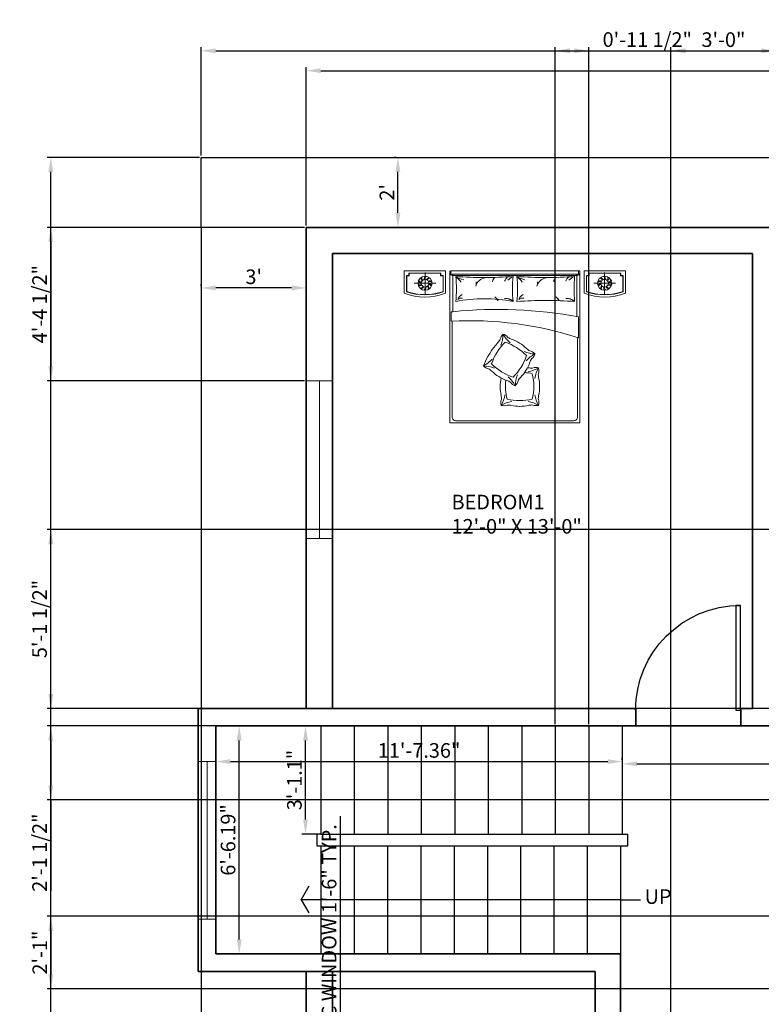
# Model space of a CAD drawing. Units: inches. Extents: x -938 to -211, y -366 to 366.
# Tile 2 of 4: x -938 to -684, y 4 to 341. Entities that reach past the tile are written whole.
import ezdxf

# ---------------------------------------------------------------- set-up
doc = ezdxf.new("R2010")
doc.units = ezdxf.units.IN
doc.header["$PDMODE"] = 35
doc.header["$PDSIZE"] = 5
for name, color, linetype, lineweight in [('A-ANNO-DIMS', 2, 'Continuous', 18), ('A-AREA-IDEN', 7, 'Continuous', 18), ('A-DOOR', 3, 'Continuous', 25), ('A-FLOR-STRS', 7, 'Continuous', 25), ('A-GLAZ', 4, 'Continuous', 18), ('A-WALL', 7, 'Continuous', 35), ('C-PROP', 8, 'Continuous', 25), ('furn', 28, 'Continuous', 13), ('txt', 7, 'Continuous', 18)]:
    doc.layers.add(name, color=color, linetype=linetype, lineweight=lineweight)
doc.styles.get("Standard").update_dxf_attribs({"font": 'arial.ttf'})
doc.dimstyles.new('ISO-25', dxfattribs={"dimtxt": 5, "dimasz": 5, "dimexe": 1.25, "dimexo": 0.625, "dimtad": 1, "dimlunit": 3, "dimtxsty": 'Standard', "dimcen": 2.5, "dimadec": 0, "dimazin": 0, "dimtfac": 1, "dimtmove": 0, "dimatfit": 3, "dimfxl": 1, "dimarcsym": 0})

# ---------------------------------------------------------------- blocks, each defined once
blk = doc.blocks.new('*U2')
for p, q in [((0, 0), (0, -6)), ((40, 0), (40, -6))]:
    blk.add_line(p, q)
blk.add_lwpolyline([(0, 0), (0, 40), (1.75, 40), (1.75, 0)], close=True)
blk.add_arc((0, 0), 40, 0, 90)
blk = doc.blocks.new('*D14')
at = {"layer": 'A-ANNO-DIMS', "color": 0, "lineweight": -2, "transparency": 16777216}
for p, q in [((-560.06, 104.36), (-560.06, 84.74)), ((-731.7, 98.36), (-731.7, 84.74)), ((-726.7, 85.99), (-565.06, 85.99))]:
    blk.add_line(p, q, dxfattribs=at)
at = {"layer": 'A-ANNO-DIMS', "color": 0, "transparency": 16777216}
for points in [[(-726.7, 86.82), (-726.7, 85.15), (-731.7, 85.99)], [(-565.06, 86.82), (-565.06, 85.15), (-560.06, 85.99)]]:
    blk.add_solid(points, dxfattribs=at)
at = {"layer": 'Defpoints', "color": 0, "transparency": 16777216}
for p in [(-560.06, 104.98), (-731.7, 98.98), (-560.06, 85.99)]:
    blk.add_point(p, dxfattribs=at)
at = {"layer": 'A-ANNO-DIMS', "color": 0, "transparency": 16777216, "insert": (-645.88, 89.17), "char_height": 5, "attachment_point": 5}
blk.add_mtext('14\'-3.64"', dxfattribs=at)
blk = doc.blocks.new('*D15')
at = {"layer": 'A-ANNO-DIMS', "color": 0, "lineweight": -2, "transparency": 16777216}
for p, q in [((-870.44, 98.98), (-861.78, 98.98)), ((-863.03, 25.79), (-863.03, 93.98)), ((-870.44, 20.79), (-861.78, 20.79))]:
    blk.add_line(p, q, dxfattribs=at)
at = {"layer": 'A-ANNO-DIMS', "color": 0, "transparency": 16777216}
for points in [[(-863.87, 93.98), (-862.2, 93.98), (-863.03, 98.98)], [(-863.87, 25.79), (-862.2, 25.79), (-863.03, 20.79)]]:
    blk.add_solid(points, dxfattribs=at)
at = {"layer": 'Defpoints', "color": 0, "transparency": 16777216}
for p in [(-871.06, 98.98), (-863.03, 98.98), (-871.06, 20.79)]:
    blk.add_point(p, dxfattribs=at)
at = {"layer": 'A-ANNO-DIMS', "color": 0, "transparency": 16777216, "insert": (-866.21, 59.89), "char_height": 5, "attachment_point": 5, "rotation": 90}
blk.add_mtext('6\'-6.19"', dxfattribs=at)
blk = doc.blocks.new('*D16')
at = {"layer": 'A-ANNO-DIMS', "color": 0, "lineweight": -2, "transparency": 16777216}
for p, q in [((-835.69, 98.98), (-841.54, 98.98)), ((-840.29, 66.89), (-840.29, 93.98)), ((-836.19, 61.89), (-841.54, 61.89))]:
    blk.add_line(p, q, dxfattribs=at)
at = {"layer": 'A-ANNO-DIMS', "color": 0, "transparency": 16777216}
for points in [[(-841.12, 93.98), (-839.46, 93.98), (-840.29, 98.98)], [(-841.12, 66.89), (-839.46, 66.89), (-840.29, 61.89)]]:
    blk.add_solid(points, dxfattribs=at)
at = {"layer": 'Defpoints', "color": 0, "transparency": 16777216}
for p in [(-840.29, 98.98), (-835.06, 98.98), (-835.56, 61.89)]:
    blk.add_point(p, dxfattribs=at)
at = {"layer": 'A-ANNO-DIMS', "color": 0, "transparency": 16777216, "insert": (-843.47, 80.43), "char_height": 5, "attachment_point": 5, "rotation": 90}
blk.add_mtext('3\'-1.1"', dxfattribs=at)
blk = doc.blocks.new('*D17')
at = {"layer": 'A-ANNO-DIMS', "color": 0, "lineweight": -2, "transparency": 16777216}
for p, q in [((-871.06, 87.39), (-871.06, 88.01)), ((-731.7, 87.39), (-731.7, 88.01)), ((-866.06, 86.76), (-736.7, 86.76))]:
    blk.add_line(p, q, dxfattribs=at)
at = {"layer": 'A-ANNO-DIMS', "color": 0, "transparency": 16777216}
for points in [[(-866.06, 87.59), (-866.06, 85.93), (-871.06, 86.76)], [(-736.7, 87.59), (-736.7, 85.93), (-731.7, 86.76)]]:
    blk.add_solid(points, dxfattribs=at)
at = {"layer": 'Defpoints', "color": 0, "transparency": 16777216}
for p in [(-871.06, 86.76), (-731.7, 86.76), (-731.7, 86.76)]:
    blk.add_point(p, dxfattribs=at)
at = {"layer": 'A-ANNO-DIMS', "color": 0, "transparency": 16777216, "insert": (-801.38, 89.94), "char_height": 5, "attachment_point": 5}
blk.add_mtext('11\'-7.36"', dxfattribs=at)
blk = doc.blocks.new('*D20')
at = {"layer": 'A-ANNO-DIMS', "color": 0, "lineweight": -2, "transparency": 16777216}
for p, q in [((-809.24, 293.98), (-809.87, 293.98)), ((-808.62, 274.98), (-808.62, 288.98)), ((-809.24, 269.98), (-809.87, 269.98))]:
    blk.add_line(p, q, dxfattribs=at)
at = {"layer": 'A-ANNO-DIMS', "color": 0, "transparency": 16777216}
for points in [[(-809.45, 288.98), (-807.78, 288.98), (-808.62, 293.98)], [(-809.45, 274.98), (-807.78, 274.98), (-808.62, 269.98)]]:
    blk.add_solid(points, dxfattribs=at)
at = {"layer": 'Defpoints', "color": 0, "transparency": 16777216}
for p in [(-808.62, 293.98), (-808.62, 293.98), (-808.62, 269.98)]:
    blk.add_point(p, dxfattribs=at)
at = {"layer": 'A-ANNO-DIMS', "color": 0, "transparency": 16777216, "insert": (-811.75, 281.98), "char_height": 5, "attachment_point": 5, "rotation": 90}
blk.add_mtext("2'", dxfattribs=at)
blk = doc.blocks.new('*D21')
at = {"layer": 'A-ANNO-DIMS', "color": 0, "lineweight": -2, "transparency": 16777216}
for p, q in [((-876.06, 249.82), (-876.06, 250.45)), ((-840.06, 249.82), (-840.06, 250.45)), ((-845.06, 249.2), (-871.06, 249.2))]:
    blk.add_line(p, q, dxfattribs=at)
at = {"layer": 'A-ANNO-DIMS', "color": 0, "transparency": 16777216}
for points in [[(-871.06, 250.03), (-871.06, 248.37), (-876.06, 249.2)], [(-845.06, 250.03), (-845.06, 248.37), (-840.06, 249.2)]]:
    blk.add_solid(points, dxfattribs=at)
at = {"layer": 'Defpoints', "color": 0, "transparency": 16777216}
for p in [(-876.06, 249.2), (-876.06, 249.2), (-840.06, 249.2)]:
    blk.add_point(p, dxfattribs=at)
at = {"layer": 'A-ANNO-DIMS', "color": 0, "transparency": 16777216, "insert": (-858.06, 252.38), "char_height": 5, "attachment_point": 5}
blk.add_mtext("3'", dxfattribs=at)
blk = doc.blocks.new('*D22')
at = {"layer": 'A-ANNO-DIMS', "color": 0, "lineweight": -2, "transparency": 16777216}
for p, q in [((-840.06, 270.61), (-840.06, 324.96)), ((-300.06, 270.61), (-300.06, 324.96)), ((-835.06, 323.71), (-305.06, 323.71))]:
    blk.add_line(p, q, dxfattribs=at)
at = {"layer": 'A-ANNO-DIMS', "color": 0, "transparency": 16777216}
for points in [[(-835.06, 324.54), (-835.06, 322.87), (-840.06, 323.71)], [(-305.06, 324.54), (-305.06, 322.87), (-300.06, 323.71)]]:
    blk.add_solid(points, dxfattribs=at)
at = {"layer": 'Defpoints', "color": 0, "transparency": 16777216}
for p in [(-300.06, 323.71), (-840.06, 269.98), (-300.06, 269.98)]:
    blk.add_point(p, dxfattribs=at)
at = {"layer": 'A-ANNO-DIMS', "color": 0, "transparency": 16777216, "insert": (-570.06, 326.87), "char_height": 5, "attachment_point": 5}
blk.add_mtext("45'", dxfattribs=at)
blk = doc.blocks.new('BED-DOUBLE-WITH-NIGHTSTANDS')
for p, q in [((-30.77, -7.97), (-30.77, -0.55)), ((-21.46, -1.59), (21.46, -1.59)), ((-21.24, -1.21), (-21.24, -14.04)), ((21.22, -1.21), (21.22, -15.71)), ((30.77, -7.97), (30.77, -0.55)), ((-34.48, -4.26), (-27.06, -4.26)), ((34.48, -4.26), (27.06, -4.26))]:
    blk.add_line(p, q)
for points in [[(-37.91, -7.71), (-37.91, 0), (-23.78, 0), (-23.78, -7.71, -0.181818)], [(-20.26, -10.53, 0.058596), (-20.26, -1.94, 0.036889), (-0.58, -1.94, 0.052163), (-0.58, -10.53, 0.093111)], [(0.7, -10.53, 0.058596), (0.7, -1.94, 0.036648), (20.51, -1.94, 0.052163), (20.51, -10.53, 0.036967)], [(37.91, -7.71), (37.91, 0), (23.78, 0), (23.78, -7.71, 0.181818)], [(-21.84, -14.04), (-21.24, -14.04, -0.072944), (21.82, -15.84), (21.82, -22.97, 0.092568), (-21.84, -17.31)]]:
    blk.add_lwpolyline(points, format="xyb", close=True)
for points in [[(-36.29, -0.77), (-36.29, -1.62), (-37.14, -1.62)], [(-36.22, -0.77), (-36.22, -1.7), (-37.14, -1.7)], [(-36.29, -0.77), (-25.39, -0.77)], [(-36.29, -0.85), (-25.39, -0.85)], [(-25.47, -0.77), (-25.47, -1.7), (-24.55, -1.7)], [(-25.39, -0.77), (-25.39, -1.62), (-24.55, -1.62)], [(-22.23, 0), (-22.23, -52.18), (22.23, -52.18), (22.23, 0)], [(21.82, 0), (21.82, -1.21), (-21.98, -1.21), (-21.98, 0), (22.23, 0)], [(25.39, -0.77), (25.39, -1.62), (24.55, -1.62)], [(25.47, -0.77), (25.47, -1.7), (24.55, -1.7)], [(36.29, -0.77), (25.39, -0.77)], [(36.29, -0.85), (25.39, -0.85)], [(36.22, -0.77), (36.22, -1.7), (37.14, -1.7)], [(36.29, -0.77), (36.29, -1.62), (37.14, -1.62)]]:
    blk.add_lwpolyline(points)
for points in [[(-24.55, -1.62), (-24.55, -7.18, -0.167087), (-37.14, -7.18), (-37.14, -1.62)], [(-24.62, -1.62), (-24.62, -7.12, -0.165559), (-37.06, -7.12), (-37.06, -1.62)], [(24.55, -1.62), (24.55, -7.17, 0.167087), (37.14, -7.17), (37.14, -1.62)], [(24.62, -1.62), (24.62, -7.12, 0.165559), (37.06, -7.12), (37.06, -1.62)], [(-21.46, -17.29), (-21.46, -50.12, 0.414214), (-20.18, -51.41), (20.18, -51.41, 0.414214), (21.46, -50.12), (21.46, -22.84)], [(-4.77, -25.48, 0.091296), (-3.99, -21.71, 0.091296), (-1.62, -24.74, 0.091296)], [(-7.96, -31.91, 0.111006), (-0.61, -36.48, 0.119549), (4.01, -29.05, 0.107813), (-3.31, -24.46)], [(-3.34, -24.47, 0.121865), (-7.96, -31.91, 0.121865)], [(-7.02, -33.41, 0.091296), (-10.79, -32.62, 0.091296), (-7.75, -30.26, 0.091296)], [(0.12, -39.42, 0.159461), (1.12, -37.65, -0.076283), (1.91, -36.55, 0.115075), (5.13, -31.37, -0.076283), (5.77, -30.18, 0.159461), (6.92, -28.51)], [(3.15, -27.72, 0.091296), (6.92, -28.51, 0.091296), (3.88, -30.87, 0.091296)], [(4.54, -34.62, 0.091296), (8.15, -33.3, 0.091296), (6.83, -36.91, 0.091296)], [(8.15, -46.15, 0.159461), (8.07, -44.13, -0.076283), (8.15, -42.78, 0.115075), (8.15, -36.68, -0.076283), (8.07, -35.33, 0.159461), (8.15, -33.3)], [(-2.67, -44.06, 0.111006), (5.98, -44.05, 0.119549), (5.98, -35.3, 0.033212), (3.32, -34.89)], [(0.9, -35.65, 0.091296), (0.12, -39.42, 0.091296), (-2.25, -36.39)], [(-1.08, -44.84, 0.091296), (-4.7, -46.15, 0.091296), (-3.37, -42.55, 0.091296)], [(6.83, -42.55, 0.091296), (8.15, -46.15, 0.091296), (4.54, -44.84)]]:
    blk.add_lwpolyline(points, format="xyb")
for centre, radius in [((-30.77, -4.26), 2.42), ((-30.77, -4.26), 1.31), ((30.77, -4.26), 2.42), ((30.77, -4.26), 1.31)]:
    blk.add_circle(centre, radius)
for centre, radius, start, end in [((-31.77, -2.78), 1.19, 196.3002, 256.538), ((-30.56, -2.45), 1.56, 172.17, 218.4897), ((-30.71, -2.48), 1.19, 160.3002, 220.538), ((-29.53, -2.92), 1.56, 136.17, 182.4897), ((-29.67, -2.86), 1.19, 124.3002, 184.538), ((-28.98, -3.9), 1.56, 100.17, 146.4897), ((-29.06, -3.77), 1.19, 88.3002, 148.538), ((-21.46, -0.82), 0.771, 180, 270), ((-15.69, 5.24), 8.51, 237.5379, 257.5233), ((-26.7, -9.98), 10.3, 36.4935, 51.2792), ((-9.16, -7.04), 4.76, 96.6849, 148.3182), ((-4.35, -4.33), 3.34, 141.8174, 169.8987), ((-0.12, -4.8), 3.6, 130.5354, 160.3558), ((2.12, -7.83), 6.48, 114.6457, 134.1585), ((-5.74, -9.98), 10.3, 36.4935, 51.2792), ((5.27, 5.24), 8.51, 237.5379, 257.5233), ((11.8, -7.04), 4.76, 96.6849, 148.3182), ((16.61, -4.33), 3.34, 141.8174, 169.8987), ((20.84, -4.8), 3.6, 130.5354, 160.3558), ((23.08, -7.83), 6.48, 114.6457, 134.1585), ((21.46, -0.82), 0.771, 270, 0), ((29.06, -3.77), 1.19, 31.462, 91.6998), ((28.98, -3.9), 1.56, 33.5103, 79.83), ((29.67, -2.86), 1.19, 355.462, 55.6998), ((29.53, -2.92), 1.56, 357.5103, 43.83), ((30.71, -2.48), 1.19, 319.462, 19.6998), ((30.73, -2.38), 1.56, 321.5103, 7.83), ((31.94, -2.72), 1.19, 283.462, 343.6998), ((31.84, -2.6), 1.56, 285.5103, 331.83), ((-32.44, -3.65), 1.19, 232.3002, 292.538), ((-32.43, -3.5), 1.56, 244.17, 290.4897), ((-31.66, -2.67), 1.56, 208.17, 254.4897), ((-32.48, -4.75), 1.19, 268.3002, 328.538), ((-32.56, -4.62), 1.56, 280.17, 326.4897), ((-31.87, -5.66), 1.19, 304.3002, 4.538), ((-32.01, -5.6), 1.56, 316.17, 2.4897), ((-30.83, -6.04), 1.19, 340.3002, 40.538), ((-30.99, -6.07), 1.56, 352.17, 38.4897), ((-29.11, -5.02), 1.56, 64.17, 110.4897), ((-29.1, -4.87), 1.19, 52.3002, 112.538), ((-29.78, -5.74), 1.19, 16.3002, 76.538), ((-29.88, -5.85), 1.56, 28.17, 74.4897), ((-15.35, -4.38), 2.13, 335.8927, 16.1192), ((5.61, -4.38), 2.13, 335.8927, 16.1192), ((29.1, -4.87), 1.19, 67.462, 127.6998), ((29.11, -5.03), 1.56, 69.5103, 115.83), ((29.88, -5.85), 1.56, 105.5103, 151.83), ((29.78, -5.74), 1.19, 103.462, 163.6998), ((30.99, -6.07), 1.56, 141.5103, 187.83), ((30.83, -6.04), 1.19, 139.462, 199.6998), ((32.01, -5.6), 1.56, 177.5103, 223.83), ((31.87, -5.66), 1.19, 175.462, 235.6998), ((32.56, -4.62), 1.56, 213.5103, 259.83), ((32.48, -4.75), 1.19, 211.462, 271.6998), ((32.61, -3.43), 1.56, 249.5103, 295.83), ((32.62, -3.58), 1.19, 247.462, 307.6998), ((-16.88, -10.73), 2.86, 114.2916, 160.9896), ((-18.36, -11.33), 1.95, 76.4823, 128.5563), ((-14.47, -16.51), 10.73, 36.2085, 45.0849), ((-6.53, -10.17), 0.72, 353.7543, 77.2187), ((-3.09, -12.99), 3.51, 44.406, 96.8342), ((-2.43, -11.76), 2.23, 33.6349, 90.8456), ((4.08, -10.73), 2.86, 114.2916, 160.9896), ((2.6, -11.33), 1.95, 76.4823, 128.5563), ((6.49, -16.51), 10.73, 36.2085, 45.0849), ((14.43, -10.17), 0.72, 353.7543, 77.2187), ((17.87, -12.99), 3.51, 44.406, 96.8342), ((18.53, -11.76), 2.23, 33.6349, 90.8456), ((-8.96, -21.45), 4.46, 315.5854, 333.0343), ((-1.79, -24.12), 3.26, 132.4658, 168.7065), ((-4.85, -24.74), 3.14, 37.2937, 74.0973), ((0.32, -19.25), 4.46, 233.2983, 250.7472), ((-5.44, -36.19), 13.43, 45.1307, 71.3884), ((15.27, -43.27), 28.15, 138.3818, 157.7644), ((7.15, -23.48), 4.46, 225.7718, 243.2208), ((4.59, -30.42), 3.01, 39.4726, 79.6505), ((-8.39, -30.41), 3.26, 222.6522, 258.8929), ((-11.03, -37.59), 4.46, 45.7718, 63.2208), ((1.73, -46.36), 13.43, 77.0576, 78.7033), ((5.69, -28.91), 4.46, 257.6988, 275.1477), ((7.19, -36.15), 3.01, 71.3996, 111.5774), ((1.56, -24.88), 13.43, 225.1307, 251.3884), ((8.38, -39.73), 13.43, 166.8711, 193.1289), ((15.01, -39.64), 18.22, 173.1956, 194.0284), ((-4.2, -41.82), 4.46, 53.2983, 70.7472), ((1.37, -35.91), 3.73, 218.7754, 250.3571), ((-9.05, -43.74), 4.46, 355.0387, 12.4877), ((-1.56, -45.28), 3.26, 159.3666, 195.6073), ((-3.83, -43.01), 3.26, 254.5791, 290.8198), ((-2.27, -50.5), 4.46, 77.6988, 95.1477), ((1.69, -33.06), 13.43, 257.0576, 283.3153), ((5.76, -50.48), 4.46, 85.2252, 102.6741), ((7.36, -42.51), 3.73, 250.7023, 282.284)]:
    blk.add_arc(centre, radius, start, end)
blk = doc.blocks.new('WINDOW-54IN')
blk.add_line((54, 0), (0, 0))
blk.add_lwpolyline([(54, 4.5), (54, -4.5), (0, -4.5), (0, 4.5)], close=True)
blk = doc.blocks.new('*D33')
at = {"layer": 'A-ANNO-DIMS', "color": 0, "lineweight": -2, "transparency": 16777216}
for p, q in [((-828.36, -15.05), (-828.36, 68.05)), ((-830.44, -15.05), (-827.11, -15.05)), ((-828.36, -28.05), (-828.36, -20.05)), ((-830.44, -33.05), (-827.11, -33.05))]:
    blk.add_line(p, q, dxfattribs=at)
at = {"layer": 'A-ANNO-DIMS', "color": 0, "transparency": 16777216}
for points in [[(-829.2, -20.05), (-827.53, -20.05), (-828.36, -15.05)], [(-829.2, -28.05), (-827.53, -28.05), (-828.36, -33.05)]]:
    blk.add_solid(points, dxfattribs=at)
at = {"layer": 'Defpoints', "color": 0, "transparency": 16777216}
for p in [(-831.06, -15.05), (-828.36, -15.05), (-831.06, -33.05)]:
    blk.add_point(p, dxfattribs=at)
at = {"layer": 'A-ANNO-DIMS', "color": 0, "transparency": 16777216, "insert": (-831.57, 29), "char_height": 5, "attachment_point": 5, "rotation": 90}
blk.add_mtext('WC WINDOW 1\'-6" TYP.', dxfattribs=at)
blk = doc.blocks.new('*D43')
at = {"layer": 'A-ANNO-DIMS', "color": 0, "lineweight": -2, "transparency": 16777216}
for p, q in [((-876.06, 294.61), (-876.06, 331.78)), ((-276.06, 294.61), (-276.06, 331.78)), ((-871.06, 330.53), (-281.06, 330.53))]:
    blk.add_line(p, q, dxfattribs=at)
at = {"layer": 'A-ANNO-DIMS', "color": 0, "transparency": 16777216}
for points in [[(-871.06, 331.37), (-871.06, 329.7), (-876.06, 330.53)], [(-281.06, 331.37), (-281.06, 329.7), (-276.06, 330.53)]]:
    blk.add_solid(points, dxfattribs=at)
at = {"layer": 'Defpoints', "color": 0, "transparency": 16777216}
for p in [(-276.06, 330.53), (-876.06, 293.98), (-276.06, 293.98)]:
    blk.add_point(p, dxfattribs=at)
at = {"layer": 'A-ANNO-DIMS', "color": 0, "transparency": 16777216, "insert": (-576.06, 333.71), "char_height": 5, "attachment_point": 5}
blk.add_mtext('50\'-0"', dxfattribs=at)
blk = doc.blocks.new('*D44')
at = {"layer": 'A-ANNO-DIMS', "color": 0, "lineweight": -2, "transparency": 16777216}
for p, q in [((-876.69, 293.98), (-928.86, 293.98)), ((-927.61, -320.02), (-927.61, 288.98)), ((-876.69, -325.02), (-928.86, -325.02))]:
    blk.add_line(p, q, dxfattribs=at)
at = {"layer": 'A-ANNO-DIMS', "color": 0, "transparency": 16777216}
for points in [[(-928.45, 288.98), (-926.78, 288.98), (-927.61, 293.98)], [(-928.45, -320.02), (-926.78, -320.02), (-927.61, -325.02)]]:
    blk.add_solid(points, dxfattribs=at)
at = {"layer": 'Defpoints', "color": 0, "transparency": 16777216}
for p in [(-927.61, 293.98), (-876.06, 293.98), (-876.06, -325.02)]:
    blk.add_point(p, dxfattribs=at)
at = {"layer": 'A-ANNO-DIMS', "color": 0, "transparency": 16777216, "insert": (-930.79, -15.52), "char_height": 5, "attachment_point": 5, "rotation": 90}
blk.add_mtext('51\'-7"', dxfattribs=at)
blk = doc.blocks.new('*D47')
at = {"layer": 'A-ANNO-DIMS', "color": 0, "lineweight": -2, "transparency": 16777216}
for p, q in [((-715.02, -44.58), (-715.02, 331.78)), ((-679.06, -44.58), (-679.06, 331.78)), ((-710.02, 330.53), (-684.06, 330.53))]:
    blk.add_line(p, q, dxfattribs=at)
at = {"layer": 'A-ANNO-DIMS', "color": 0, "transparency": 16777216}
for points in [[(-710.02, 331.37), (-710.02, 329.7), (-715.02, 330.53)], [(-684.06, 331.37), (-684.06, 329.7), (-679.06, 330.53)]]:
    blk.add_solid(points, dxfattribs=at)
at = {"layer": 'Defpoints', "color": 0, "transparency": 16777216}
for p in [(-679.06, 330.53), (-715.02, -45.21), (-679.06, -45.21)]:
    blk.add_point(p, dxfattribs=at)
at = {"layer": 'A-ANNO-DIMS', "color": 0, "transparency": 16777216, "insert": (-697.04, 333.71), "char_height": 5, "attachment_point": 5}
blk.add_mtext('3\'-0"', dxfattribs=at)
blk = doc.blocks.new('*D55')
at = {"layer": 'A-ANNO-DIMS', "color": 0, "lineweight": -2, "transparency": 16777216}
for p, q in [((-840.69, 269.98), (-928.86, 269.98)), ((-927.61, 264.98), (-927.61, 222.31)), ((-840.69, 217.31), (-928.86, 217.31))]:
    blk.add_line(p, q, dxfattribs=at)
at = {"layer": 'A-ANNO-DIMS', "color": 0, "transparency": 16777216}
for points in [[(-928.45, 264.98), (-926.78, 264.98), (-927.61, 269.98)], [(-928.45, 222.31), (-926.78, 222.31), (-927.61, 217.31)]]:
    blk.add_solid(points, dxfattribs=at)
at = {"layer": 'Defpoints', "color": 0, "transparency": 16777216}
for p in [(-840.06, 269.98), (-927.61, 217.31), (-840.06, 217.31)]:
    blk.add_point(p, dxfattribs=at)
at = {"layer": 'A-ANNO-DIMS', "color": 0, "transparency": 16777216, "insert": (-930.82, 243.64), "char_height": 5, "attachment_point": 5, "rotation": 90}
blk.add_mtext('4\'-4 1/2"', dxfattribs=at)
blk = doc.blocks.new('*D56')
at = {"layer": 'A-ANNO-DIMS', "color": 0, "lineweight": -2, "transparency": 16777216}
for p, q in [((-309.69, 166.31), (-928.86, 166.31)), ((-927.61, 109.98), (-927.61, 161.31)), ((-309.69, 104.98), (-928.86, 104.98))]:
    blk.add_line(p, q, dxfattribs=at)
at = {"layer": 'A-ANNO-DIMS', "color": 0, "transparency": 16777216}
for points in [[(-928.45, 161.31), (-926.78, 161.31), (-927.61, 166.31)], [(-928.45, 109.98), (-926.78, 109.98), (-927.61, 104.98)]]:
    blk.add_solid(points, dxfattribs=at)
at = {"layer": 'Defpoints', "color": 0, "transparency": 16777216}
for p in [(-927.61, 166.31), (-309.06, 166.31), (-309.06, 104.98)]:
    blk.add_point(p, dxfattribs=at)
at = {"layer": 'A-ANNO-DIMS', "color": 0, "transparency": 16777216, "insert": (-930.82, 135.65), "char_height": 5, "attachment_point": 5, "rotation": 90}
blk.add_mtext('5\'-1 1/2"', dxfattribs=at)
blk = doc.blocks.new('*D60')
at = {"layer": 'A-ANNO-DIMS', "color": 0, "lineweight": -2, "transparency": 16777216}
for p, q in [((-394.97, 33.71), (-928.86, 33.71)), ((-927.61, 28.71), (-927.61, 13.79)), ((-418.97, 8.79), (-928.86, 8.79))]:
    blk.add_line(p, q, dxfattribs=at)
at = {"layer": 'A-ANNO-DIMS', "color": 0, "transparency": 16777216}
for points in [[(-928.45, 28.71), (-926.78, 28.71), (-927.61, 33.71)], [(-928.45, 13.79), (-926.78, 13.79), (-927.61, 8.79)]]:
    blk.add_solid(points, dxfattribs=at)
at = {"layer": 'Defpoints', "color": 0, "transparency": 16777216}
for p in [(-394.34, 33.71), (-927.61, 8.79), (-418.34, 8.79)]:
    blk.add_point(p, dxfattribs=at)
at = {"layer": 'A-ANNO-DIMS', "color": 0, "transparency": 16777216, "insert": (-930.75, 21.25), "char_height": 5, "attachment_point": 5, "rotation": 90}
blk.add_mtext('2\'-1"', dxfattribs=at)
blk = doc.blocks.new('*D62')
at = {"layer": 'A-ANNO-DIMS', "color": 0, "lineweight": -2, "transparency": 16777216}
for p, q in [((-754.67, 99.61), (-754.67, 331.78)), ((-743.19, 99.61), (-743.19, 331.78)), ((-749.67, 330.53), (-748.19, 330.53)), ((-743.19, 330.53), (-708.11, 330.53))]:
    blk.add_line(p, q, dxfattribs=at)
at = {"layer": 'A-ANNO-DIMS', "color": 0, "transparency": 16777216}
for points in [[(-749.67, 331.37), (-749.67, 329.7), (-754.67, 330.53)], [(-748.19, 331.37), (-748.19, 329.7), (-743.19, 330.53)]]:
    blk.add_solid(points, dxfattribs=at)
at = {"layer": 'Defpoints', "color": 0, "transparency": 16777216}
for p in [(-743.19, 330.53), (-754.67, 98.98), (-743.19, 98.98)]:
    blk.add_point(p, dxfattribs=at)
at = {"layer": 'A-ANNO-DIMS', "color": 0, "transparency": 16777216, "insert": (-723.15, 333.74), "char_height": 5, "attachment_point": 5}
blk.add_mtext('0\'-11 1/2"', dxfattribs=at)
blk = doc.blocks.new('*D66')
at = {"layer": 'A-ANNO-DIMS', "color": 0, "lineweight": -2, "transparency": 16777216}
for p, q in [((-309.69, 98.98), (-928.86, 98.98)), ((-927.61, 93.98), (-927.61, 78.67)), ((-309.69, 73.67), (-928.86, 73.67)), ((-927.61, 73.67), (-927.61, 42.39))]:
    blk.add_line(p, q, dxfattribs=at)
at = {"layer": 'A-ANNO-DIMS', "color": 0, "transparency": 16777216}
for points in [[(-928.45, 93.98), (-926.78, 93.98), (-927.61, 98.98)], [(-928.45, 78.67), (-926.78, 78.67), (-927.61, 73.67)]]:
    blk.add_solid(points, dxfattribs=at)
at = {"layer": 'Defpoints', "color": 0, "transparency": 16777216}
for p in [(-309.06, 98.98), (-927.61, 73.67), (-309.06, 73.67)]:
    blk.add_point(p, dxfattribs=at)
at = {"layer": 'A-ANNO-DIMS', "color": 0, "transparency": 16777216, "insert": (-930.82, 55.53), "char_height": 5, "attachment_point": 5, "rotation": 90}
blk.add_mtext('2\'-1 1/2"', dxfattribs=at)

msp = doc.modelspace()

# ---------------------------------------------------------------- linework, layer by layer
at = {"layer": 'A-FLOR-STRS'}
for p, q in [((-835.062, 98.982), (-835.062, 61.887)), ((-823.578, 98.982), (-823.578, 61.887)), ((-812.093, 98.982), (-812.093, 61.887)), ((-800.609, 98.982), (-800.609, 61.887)), ((-789.124, 98.982), (-789.124, 61.887)), ((-777.64, 98.982), (-777.64, 61.887)), ((-766.155, 98.982), (-766.155, 61.887)), ((-754.67, 98.982), (-754.67, 61.887)), ((-743.186, 98.982), (-743.186, 61.887)), ((-731.701, 98.982), (-731.701, 61.887)), ((-835.062, 61.887), (-836.394, 61.887)), ((-836.394, 61.887), (-836.394, 57.908)), ((-835.062, 61.887), (-729.838, 61.887)), ((-729.838, 57.887), (-729.838, 61.887)), ((-836.394, 57.908), (-835.062, 57.887)), ((-835.062, 57.887), (-729.838, 57.887)), ((-835.062, 57.887), (-835.062, 20.791)), ((-823.644, 57.887), (-823.644, 20.791)), ((-812.225, 57.887), (-812.225, 20.791)), ((-800.807, 57.887), (-800.807, 20.791)), ((-789.388, 57.887), (-789.388, 20.791)), ((-777.97, 57.887), (-777.97, 20.791)), ((-766.551, 57.887), (-766.551, 20.791)), ((-755.133, 57.887), (-755.133, 20.791)), ((-743.714, 57.887), (-743.714, 20.791)), ((-732.296, 57.887), (-732.296, 20.791)), ((-841.762, 39.339), (-838.999, 44.125)), ((-732.296, 39.339), (-841.762, 39.339)), ((-841.762, 39.339), (-839.203, 34.906)), ((-732.296, 39.339), (-725.474, 39.339))]:
    msp.add_line(p, q, dxfattribs=at)
at = {"layer": 'A-GLAZ'}
msp.add_line((-874.062, 86.76), (-874.062, 32.76), dxfattribs=at)
msp.add_lwpolyline([(-877.062, 86.76), (-871.062, 86.76), (-871.062, 32.76), (-877.062, 32.76)], close=True, dxfattribs=at)
at = {"layer": 'A-WALL'}
for p, q in [((-840.062, 104.982), (-840.062, 269.982)), ((-840.062, 269.982), (-300.062, 269.982)), ((-831.062, 260.982), (-687.062, 260.982)), ((-831.062, 104.982), (-831.062, 260.982)), ((-687.062, 104.982), (-687.062, 260.982)), ((-840.062, 104.982), (-877.062, 104.982)), ((-877.062, 104.791), (-877.062, 104.982)), ((-877.062, 98.791), (-877.062, 104.791)), ((-831.062, 104.982), (-840.062, 104.982)), ((-831.062, 104.982), (-727.062, 104.982)), ((-727.062, 104.982), (-727.062, 98.982)), ((-691.062, 104.982), (-691.062, 98.982)), ((-691.062, 104.982), (-687.062, 104.982)), ((-877.062, 98.791), (-877.062, 14.791)), ((-871.062, 98.982), (-871.062, 20.791)), ((-840.062, 98.982), (-871.062, 98.982)), ((-831.062, 98.982), (-840.062, 98.982)), ((-831.062, 98.982), (-554.062, 98.982)), ((-871.062, 20.791), (-735.062, 20.791)), ((-732.296, 20.791), (-735.062, 20.791)), ((-732.296, 20.791), (-732.296, -45.209)), ((-871.062, 14.791), (-877.062, 14.791)), ((-871.062, 14.791), (-741.062, 14.791)), ((-840.062, -270.018), (-840.062, 14.791)), ((-831.062, -51.209), (-831.062, 14.791)), ((-741.062, 14.791), (-741.062, -45.209))]:
    msp.add_line(p, q, dxfattribs=at)
at = {"layer": 'C-PROP'}
for p, q in [((-876.062, 293.982), (-300.062, 293.982)), ((-876.062, 269.982), (-876.062, 293.982)), ((-876.062, 269.982), (-876.062, -325.018))]:
    msp.add_line(p, q, dxfattribs=at)

# ---------------------------------------------------------------- block references
at = {"layer": 'A-DOOR', "xscale": -0.8986880990233336, "yscale": 0.8986880990233336, "zscale": 0.8986880990233336}
msp.add_blockref('*U2', (-691.214, 104.374), dxfattribs=at)
at = {"layer": 'A-GLAZ', "rotation": 90.00000000000011}
msp.add_blockref('WINDOW-54IN', (-835.562, 163.306), dxfattribs=at)
at = {"layer": 'furn'}
msp.add_blockref('BED-DOUBLE-WITH-NIGHTSTANDS', (-768.552, 255.079), dxfattribs=at)

# ---------------------------------------------------------------- texts
at = {"layer": 'A-AREA-IDEN', "insert": (-790.256, 178.272), "char_height": 5, "attachment_point": 1}
msp.add_mtext_dynamic_manual_height_columns('BEDROM1\\P12\'-0" X 13\'-0"', width=101.20509, gutter_width=12.5, heights=[0], dxfattribs=at)
at = {"layer": 'txt', "insert": (-724.072, 42.957), "char_height": 5, "attachment_point": 1}
msp.add_mtext_dynamic_manual_height_columns('UP', width=15.7169, gutter_width=12.5, heights=[0], dxfattribs=at)

# ---------------------------------------------------------------- dimensions: what is measured, and where the dimension line sits
at = {"layer": 'A-ANNO-DIMS'}
for base, p1, p2, override, picture, middle in [((-743.186, 330.532), (-754.67, 98.982), (-743.186, 98.982), {"dimdec": 1, "dimlfac": 1, "dimrnd": 0, "dimzin": 1, "dimdsep": 46, "dimlunit": 4, "dimfrac": 2}, '*D62', (-723.148, 333.742)), ((-276.062, 330.532), (-876.062, 293.982), (-276.062, 293.982), {"dimdec": 1, "dimlfac": 1, "dimrnd": 0, "dimzin": 1, "dimdsep": 46, "dimlunit": 4, "dimfrac": 2}, '*D43', (-576.062, 333.71)), ((-679.062, 330.532), (-715.024, -45.209), (-679.062, -45.209), {"dimdec": 1, "dimlfac": 1, "dimrnd": 0, "dimzin": 1, "dimdsep": 46, "dimlunit": 4, "dimfrac": 2}, '*D47', (-697.043, 333.711)), ((-300.062, 323.707), (-840.062, 269.982), (-300.062, 269.982), {"dimclrd": 0, "dimclre": 0, "dimclrt": 0}, '*D22', (-570.062, 326.874)), ((-876.062, 249.2), (-840.062, 249.2), (-876.062, 249.2), {"dimclrd": 0, "dimclre": 0, "dimclrt": 0}, '*D21', (-858.062, 252.38)), ((-560.062, 85.986), (-731.701, 98.982), (-560.062, 104.982), {"dimclrd": 0, "dimclre": 0, "dimclrt": 0}, '*D14', (-645.882, 89.166)), ((-731.701, 86.76), (-871.062, 86.76), (-731.701, 86.76), {"dimclrd": 0, "dimclre": 0, "dimclrt": 0}, '*D17', (-801.382, 89.94))]:
    dim = msp.add_linear_dim(base=base, p1=p1, p2=p2, dimstyle='ISO-25', override=override, dxfattribs=at)
    dim.commit()
    dim.dimension.update_dxf_attribs({"geometry": picture, "text_midpoint": middle})
for base, p1, p2, override, picture, middle in [((-927.612, 293.982), (-876.062, -325.018), (-876.062, 293.982), {"dimdec": 1, "dimlfac": 1, "dimrnd": 0, "dimzin": 1, "dimdsep": 46, "dimlunit": 4, "dimfrac": 2}, '*D44', (-930.79, -15.518)), ((-808.617, 293.982), (-808.617, 269.982), (-808.617, 293.982), {"dimclrd": 0, "dimclre": 0, "dimclrt": 0}, '*D20', (-811.752, 281.982)), ((-927.612, 217.306), (-840.062, 269.982), (-840.062, 217.306), {"dimdec": 1, "dimlfac": 1, "dimrnd": 0, "dimzin": 1, "dimdsep": 46, "dimlunit": 4, "dimfrac": 2}, '*D55', (-930.823, 243.644)), ((-927.612, 166.311), (-309.062, 104.982), (-309.062, 166.311), {"dimdec": 1, "dimlfac": 1, "dimrnd": 0, "dimzin": 1, "dimdsep": 46, "dimlunit": 4, "dimfrac": 2}, '*D56', (-930.823, 135.646)), ((-927.612, 73.669), (-309.062, 98.982), (-309.062, 73.669), {"dimdec": 1, "dimlfac": 1, "dimrnd": 0, "dimzin": 1, "dimdsep": 46, "dimlunit": 4, "dimfrac": 2}, '*D66', (-930.823, 55.531)), ((-863.033, 98.982), (-871.062, 20.791), (-871.062, 98.982), {"dimclrd": 0, "dimclre": 0, "dimclrt": 0}, '*D15', (-866.211, 59.887)), ((-840.2891, 98.9819), (-835.5624, 61.8866), (-835.0624, 98.9819), {"dimclrd": 0, "dimclre": 0, "dimclrt": 0}, '*D16', (-843.4687, 80.4342)), ((-927.612, 8.791), (-394.341, 33.709), (-418.341, 8.791), {"dimdec": 1, "dimlfac": 1, "dimrnd": 0, "dimzin": 1, "dimdsep": 46, "dimlunit": 4, "dimfrac": 2}, '*D60', (-930.748, 21.25))]:
    dim = msp.add_linear_dim(base=base, p1=p1, p2=p2, angle=90, dimstyle='ISO-25', override=override, dxfattribs=at)
    dim.commit()
    dim.dimension.update_dxf_attribs({"geometry": picture, "text_midpoint": middle})
dim = msp.add_linear_dim(base=(-828.362, -15.049), p1=(-831.062, -33.049), p2=(-831.062, -15.049), angle=90, text='WC WINDOW <> TYP.', dimstyle='ISO-25', override={"dimdec": 1, "dimlfac": 1, "dimrnd": 0, "dimzin": 1, "dimdsep": 46, "dimlunit": 4, "dimfrac": 2}, dxfattribs=at)
dim.commit()
dim.dimension.update_dxf_attribs({"geometry": '*D33', "text_midpoint": (-831.574, 29)})

doc.saveas('drawing.dxf')
